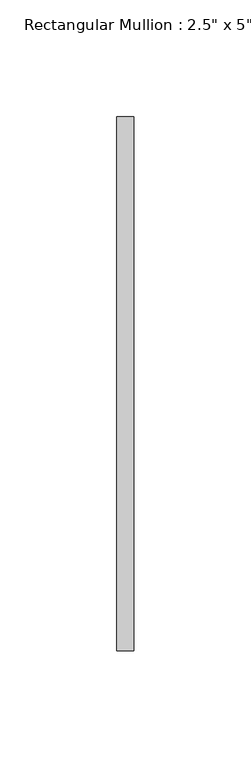
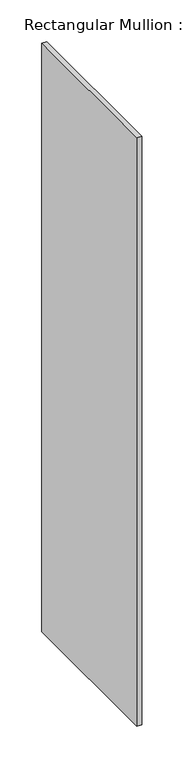
"""IFC4 building model written with IfcOpenShell, lengths in millimetres: member geometry."""

from ifc_helpers import new_model, si_unit, frame, origin, place, context, project, spatial, polyline, outline, extrude, source, transform, mapped, element, save


def member_a87dc375(model_context):
    return source(origin(), model_context, "Body", "SweptSolid", [
        extrude(outline(polyline([(3.6195, 114.3), (3.6195, -114.3), (-3.6195, -114.3), (-3.6195, 114.3), (3.6195, 114.3)])), frame((0.0, 0.0, -863.6), z_axis=(0.0, 0.0, 1.0), x_axis=(1.0, 0.0, 0.0)), (0.0, 0.0, 1.0), 863.6),
    ])


if __name__ == "__main__":
    model = new_model("IFC4")
    model_context = context("Model", 3, world=origin())
    ifc_project = project(units=[si_unit("LENGTHUNIT", "METRE", prefix="MILLI")], contexts=[model_context])
    site = spatial("IfcSite", under=ifc_project)
    building = spatial("IfcBuilding", under=site)
    placement = place(None, origin())
    member_shape = member_a87dc375(model_context)
    element("IfcMember", 1, ObjectType="Rectangular Mullion : 2.5\" x 5\" rectangular", at=placement, inside=building, context=model_context, shape_type="MappedRepresentation", body=[
        mapped(member_shape, transform((0.0, 0.0, 0.0), x_axis=(1.0, 0.0, 0.0), y_axis=(0.0, 1.0, 0.0), z_axis=(0.0, 0.0, 1.0))),
    ])
    save(model, "model.ifc")

# Revit data of these elements
# Type "Rectangular Mullion : 2.5\" x 5\" rectangular"
#   built-in parameter 1007304 = 0.75 (stored number, unit not read)
#   built-in parameter 1007301 = 0.011875 (stored number, unit not read)
#   built-in parameter 1007300 = 0.011875 (stored number, unit not read)
# Element 1 (IfcMember, "Rectangular Mullion : 2.5\" x 5\" rectangular")
#   Materials on its faces: "WINDOW GLASS MATERIAL"
# Materials
#   "WINDOW GLASS MATERIAL": class "Generic", colour RGB 120 120 120, transparency 0, Cost = 0
